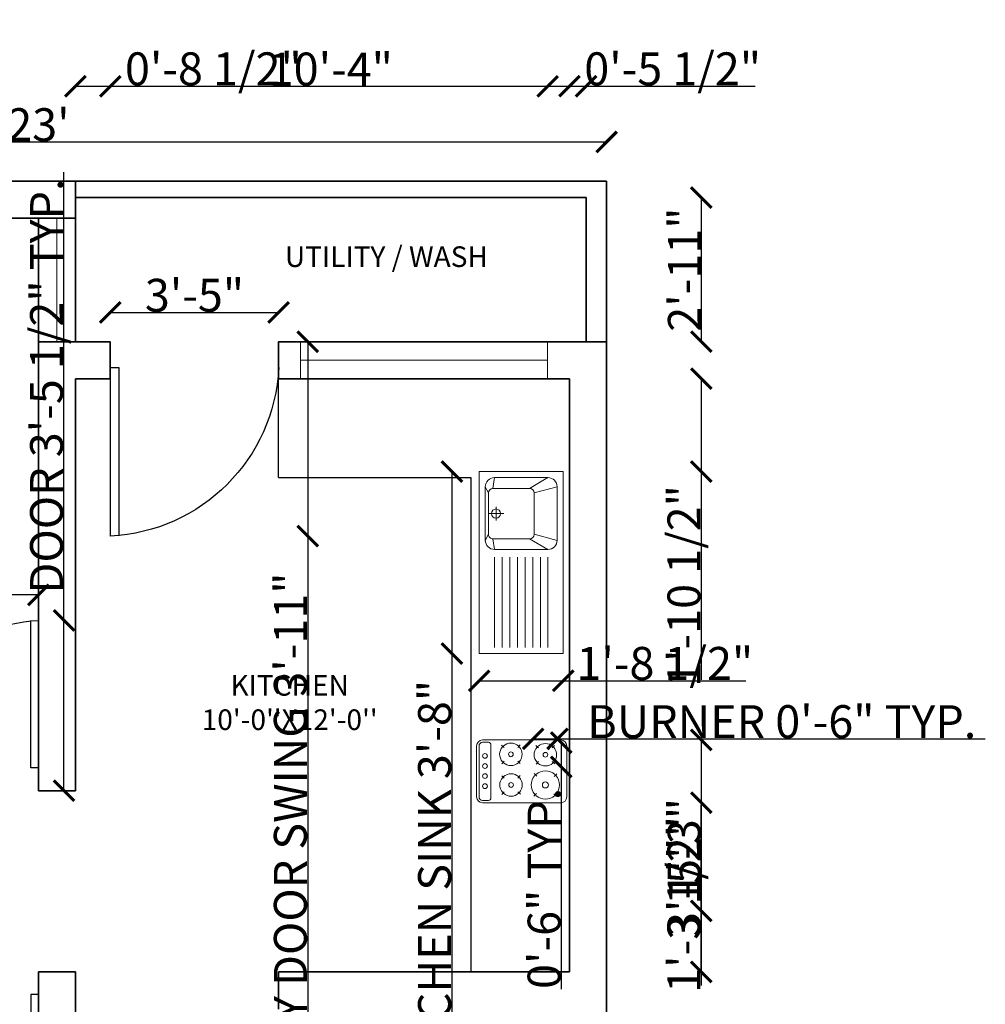
# Model space of a CAD drawing. Units: inches. Extents: x 2435 to 2891, y 1790 to 2334.
# Tile 3 of 3: x 2657 to 2891, y 2052 to 2291. Entities that reach past the tile are written whole.
import ezdxf

# ---------------------------------------------------------------- set-up
doc = ezdxf.new("R2010")
doc.units = ezdxf.units.IN
for name, color, linetype, lineweight in [('A-ANNO-DIMS', 2, 'Continuous', 13), ('A-AREA-IDEN', 7, 'Continuous', 18), ('A-EQPM', 8, 'Continuous', 13), ('A-FLOR-FIXT', 9, 'Continuous', 18), ('DOOR', 30, 'Continuous', 25), ('KITCHEN', 70, 'Continuous', 25), ('WALL', 7, 'Continuous', 35), ('WINDOW', 170, 'Continuous', 18)]:
    doc.layers.add(name, color=color, linetype=linetype, lineweight=lineweight)
doc.styles.get("Standard").update_dxf_attribs({"font": 'arial.ttf'})
doc.dimstyles.get("Standard").update_dxf_attribs({"dimtxt": 8, "dimasz": 5, "dimexe": 0.18, "dimexo": 0.0625, "dimgap": 0.09, "dimtad": 1, "dimdec": 1, "dimzin": 0, "dimdsep": 46, "dimlunit": 4, "dimtxsty": 'Standard', "dimblk": 'ARCHTICK', "dimcen": 0.09, "dimse1": 1, "dimse2": 1, "dimadec": 0, "dimazin": 0, "dimtfac": 1, "dimtdec": 1, "dimtofl": 0, "dimtmove": 0, "dimatfit": 3, "dimfxl": 1, "dimtolj": 1, "dimtzin": 0, "dimarcsym": 0})

# ---------------------------------------------------------------- blocks, each defined once
blk = doc.blocks.new('KK')
for p, q in [((0, 0.55), (0, 0)), ((1.19, 0.55), (0, 0.55)), ((1.19, 0), (1.19, 0.55)), ((0.1, 0.51), (0.14, 0.36)), ((0.45, 0.51), (0.1, 0.51)), ((0.41, 0.36), (0.45, 0.51)), ((0.11, 0.33), (0.04, 0.45)), ((0.04, 0.45), (0.04, 0.1)), ((0.44, 0.33), (0.51, 0.45)), ((0.51, 0.1), (0.51, 0.45)), ((0.56, 0.45), (1.15, 0.45)), ((0.56, 0.4), (1.15, 0.4)), ((0.11, 0.09), (0.11, 0.33)), ((0.14, 0.36), (0.41, 0.36)), ((0.44, 0.33), (0.44, 0.09)), ((0.56, 0.35), (1.15, 0.35)), ((0.56, 0.3), (1.15, 0.3)), ((0.56, 0.25), (1.15, 0.25)), ((0.56, 0.2), (1.15, 0.2)), ((0.275, 0.06), (0.275, 0.16)), ((0.56, 0.15), (1.15, 0.15)), ((0.04, 0.1), (0.11, 0.09)), ((0.23, 0.11), (0.32, 0.11)), ((0.44, 0.09), (0.51, 0.1)), ((0.56, 0.1), (1.15, 0.1)), ((0, 0), (1.19, 0)), ((0.14, 0.06), (0.1, 0.04)), ((0.1, 0.04), (0.45, 0.04)), ((0.41, 0.06), (0.14, 0.06)), ((0.41, 0.06), (0.45, 0.04))]:
    blk.add_line(p, q)
blk.add_circle((0.275, 0.11), 0.03)
for centre, radius, start, end in [((0.1, 0.45), 0.06, 90, 180), ((0.45, 0.45), 0.06, 0, 90), ((0.14, 0.33), 0.03, 90, 180), ((0.41, 0.33), 0.03, 0, 90), ((0.1, 0.1), 0.06, 180, 270), ((0.14, 0.09), 0.03, 180, 270), ((0.41, 0.09), 0.03, 270, 0), ((0.45, 0.1), 0.06, 270, 0)]:
    blk.add_arc(centre, radius, start, end)
blk = doc.blocks.new('AP0B05')
for p, q in [((35, 100), (35, 880)), ((75, 100), (75, 878.9)), ((35, 100), (35, -20)), ((815, 100), (815, -20))]:
    blk.add_line(p, q)
blk.add_lwpolyline([(35, 100), (75, 100)])
blk.add_arc((-2.4, 62.6), 818.3, 2.6212, 87.3788)
blk = doc.blocks.new('_ArchTick')
at = {"color": 0, "linetype": 'ByBlock', "const_width": 0.15}
blk.add_lwpolyline([(-0.5, -0.5), (0.5, 0.5)], dxfattribs=at)
blk = doc.blocks.new('*D10')
at = {"layer": 'A-ANNO-DIMS', "color": 0, "lineweight": -2, "transparency": 16777216}
blk.add_line((2523.44, 2261.69), (2799.44, 2261.69), dxfattribs=at)
at = {"layer": 'Defpoints', "color": 0, "transparency": 16777216}
for p in [(2799.44, 2261.69), (2523.44, 2252.2), (2799.44, 2252.2)]:
    blk.add_point(p, dxfattribs=at)
at = {"layer": 'A-ANNO-DIMS', "color": 0, "lineweight": -2, "transparency": 16777216, "xscale": 5, "yscale": 5, "zscale": 5, "rotation": 180}
blk.add_blockref('_ArchTick', (2523.44, 2261.69), dxfattribs=at)
at = {"layer": 'A-ANNO-DIMS', "color": 0, "lineweight": -2, "transparency": 16777216, "xscale": 5, "yscale": 5, "zscale": 5}
blk.add_blockref('_ArchTick', (2799.44, 2261.69), dxfattribs=at)
at = {"layer": 'A-ANNO-DIMS', "color": 0, "transparency": 16777216, "insert": (2661.44, 2265.87), "char_height": 8, "attachment_point": 5}
blk.add_mtext("\\A1;23'", dxfattribs=at)
blk = doc.blocks.new('WIN-60IN')
blk.add_line((0, 4.5), (60, 4.5))
blk.add_lwpolyline([(0, 9), (60, 9), (60, 0), (0, 0)], close=True)
blk = doc.blocks.new('COOKTOP-BURNER')
for p, q in [((-2.28, 2.23), (-1.67, 1.66)), ((2.23, 2.28), (1.66, 1.67)), ((-2.23, -2.28), (-1.66, -1.67)), ((2.28, -2.23), (1.67, -1.66))]:
    blk.add_line(p, q)
blk.add_circle((0, 0), 0.576)
for start, end in [(48.017, 131.983), (138.017, 221.983), (318.017, 41.983), (228.017, 311.983)]:
    blk.add_arc((0, 0), 2.73, start, end)
blk = doc.blocks.new('*D15')
at = {"layer": 'A-ANNO-DIMS', "color": 0, "lineweight": -2, "transparency": 16777216}
for p, q in [((2667.64, 2145.53), (2667.64, 2254.35)), ((2667.64, 2104.2), (2667.64, 2145.53))]:
    blk.add_line(p, q, dxfattribs=at)
at = {"layer": 'Defpoints', "color": 0, "transparency": 16777216}
for p in [(2661.44, 2145.53), (2667.64, 2145.53), (2661.44, 2104.2)]:
    blk.add_point(p, dxfattribs=at)
at = {"layer": 'A-ANNO-DIMS', "color": 0, "lineweight": -2, "transparency": 16777216, "xscale": 5, "yscale": 5, "zscale": 5}
for p, rotation in [((2667.64, 2145.53), 90), ((2667.64, 2104.2), 270)]:
    blk.add_blockref('_ArchTick', p, dxfattribs=dict(at, rotation=rotation))
at = {"layer": 'A-ANNO-DIMS', "color": 0, "transparency": 16777216, "insert": (2663.41, 2202.44), "char_height": 8, "attachment_point": 5, "rotation": 90}
blk.add_mtext('\\A1;DOOR 3\'-5 1/2" TYP.', dxfattribs=at)
blk = doc.blocks.new('*D16')
at = {"layer": 'A-ANNO-DIMS', "color": 0, "lineweight": -2, "transparency": 16777216}
for p, q in [((2625.63, 2151.73), (2571.69, 2151.73)), ((2661.44, 2151.73), (2625.63, 2151.73))]:
    blk.add_line(p, q, dxfattribs=at)
at = {"layer": 'Defpoints', "color": 0, "transparency": 16777216}
for p in [(2625.63, 2151.73), (2625.63, 2145.53), (2661.44, 2145.53)]:
    blk.add_point(p, dxfattribs=at)
at = {"layer": 'A-ANNO-DIMS', "color": 0, "lineweight": -2, "transparency": 16777216, "xscale": 5, "yscale": 5, "zscale": 5, "rotation": 180}
blk.add_blockref('_ArchTick', (2625.63, 2151.73), dxfattribs=at)
at = {"layer": 'A-ANNO-DIMS', "color": 0, "lineweight": -2, "transparency": 16777216, "xscale": 5, "yscale": 5, "zscale": 5}
blk.add_blockref('_ArchTick', (2661.44, 2151.73), dxfattribs=at)
at = {"layer": 'A-ANNO-DIMS', "color": 0, "transparency": 16777216, "insert": (2596.16, 2155.91), "char_height": 8, "attachment_point": 5}
blk.add_mtext('\\A1;3\'-0" TYP.', dxfattribs=at)
blk = doc.blocks.new('*D17')
at = {"layer": 'A-ANNO-DIMS', "color": 0, "lineweight": -2, "transparency": 16777216}
for p, q in [((2726.86, 2213.2), (2726.86, 2166.02)), ((2726.86, 2166.02), (2726.86, 2011.45))]:
    blk.add_line(p, q, dxfattribs=at)
at = {"layer": 'Defpoints', "color": 0, "transparency": 16777216}
for p in [(2719.78, 2213.2), (2719.78, 2166.02), (2726.86, 2166.02)]:
    blk.add_point(p, dxfattribs=at)
at = {"layer": 'A-ANNO-DIMS', "color": 0, "lineweight": -2, "transparency": 16777216, "xscale": 5, "yscale": 5, "zscale": 5}
for p, rotation in [((2726.86, 2213.2), 90), ((2726.86, 2166.02), 270)]:
    blk.add_blockref('_ArchTick', p, dxfattribs=dict(at, rotation=rotation))
at = {"layer": 'A-ANNO-DIMS', "color": 0, "transparency": 16777216, "insert": (2722.63, 2086.24), "char_height": 8, "attachment_point": 5, "rotation": 90}
blk.add_mtext('\\A1;UTILITY DOOR SWING 3\'-11"', dxfattribs=at)
blk = doc.blocks.new('*D18')
at = {"layer": 'A-ANNO-DIMS', "color": 0, "lineweight": -2, "transparency": 16777216}
blk.add_line((2678.89, 2220.28), (2719.78, 2220.28), dxfattribs=at)
at = {"layer": 'Defpoints', "color": 0, "transparency": 16777216}
for p in [(2719.78, 2220.28), (2678.89, 2213.2), (2719.78, 2213.2)]:
    blk.add_point(p, dxfattribs=at)
at = {"layer": 'A-ANNO-DIMS', "color": 0, "lineweight": -2, "transparency": 16777216, "xscale": 5, "yscale": 5, "zscale": 5, "rotation": 180}
blk.add_blockref('_ArchTick', (2678.89, 2220.28), dxfattribs=at)
at = {"layer": 'A-ANNO-DIMS', "color": 0, "lineweight": -2, "transparency": 16777216, "xscale": 5, "yscale": 5, "zscale": 5}
blk.add_blockref('_ArchTick', (2719.78, 2220.28), dxfattribs=at)
at = {"layer": 'A-ANNO-DIMS', "color": 0, "transparency": 16777216, "insert": (2699.34, 2224.46), "char_height": 8, "attachment_point": 5}
blk.add_mtext('\\A1;3\'-5"', dxfattribs=at)
blk = doc.blocks.new('*D29')
at = {"layer": 'A-ANNO-DIMS', "color": 0, "lineweight": -2, "transparency": 16777216}
for p, q in [((2781.61, 2116.78), (2787.54, 2116.78)), ((2787.54, 2116.78), (2891.43, 2116.78))]:
    blk.add_line(p, q, dxfattribs=at)
at = {"layer": 'Defpoints', "color": 0, "transparency": 16777216}
for p in [(2781.61, 2115.89), (2787.54, 2116.78), (2787.54, 2115.89)]:
    blk.add_point(p, dxfattribs=at)
at = {"layer": 'A-ANNO-DIMS', "color": 0, "lineweight": -2, "transparency": 16777216, "xscale": 5, "yscale": 5, "zscale": 5, "rotation": 180}
blk.add_blockref('_ArchTick', (2781.61, 2116.78), dxfattribs=at)
at = {"layer": 'A-ANNO-DIMS', "color": 0, "lineweight": -2, "transparency": 16777216, "xscale": 5, "yscale": 5, "zscale": 5}
blk.add_blockref('_ArchTick', (2787.54, 2116.78), dxfattribs=at)
at = {"layer": 'A-ANNO-DIMS', "color": 0, "transparency": 16777216, "insert": (2841.99, 2120.96), "char_height": 8, "attachment_point": 5}
blk.add_mtext('\\A1;BURNER 0\'-6" TYP.', dxfattribs=at)
blk = doc.blocks.new('*D30')
at = {"layer": 'A-ANNO-DIMS', "color": 0, "lineweight": -2, "transparency": 16777216}
for p, q in [((2788.43, 2115.89), (2788.43, 2109.96)), ((2788.43, 2109.96), (2788.43, 2056.01))]:
    blk.add_line(p, q, dxfattribs=at)
at = {"layer": 'Defpoints', "color": 0, "transparency": 16777216}
for p in [(2787.54, 2115.89), (2787.54, 2109.96), (2788.43, 2109.96)]:
    blk.add_point(p, dxfattribs=at)
at = {"layer": 'A-ANNO-DIMS', "color": 0, "lineweight": -2, "transparency": 16777216, "xscale": 5, "yscale": 5, "zscale": 5}
for p, rotation in [((2788.43, 2115.89), 90), ((2788.43, 2109.96), 270)]:
    blk.add_blockref('_ArchTick', p, dxfattribs=dict(at, rotation=rotation))
at = {"layer": 'A-ANNO-DIMS', "color": 0, "transparency": 16777216, "insert": (2784.26, 2080.49), "char_height": 8, "attachment_point": 5, "rotation": 90}
blk.add_mtext('\\A1;0\'-6" TYP.', dxfattribs=at)
blk = doc.blocks.new('*D31')
at = {"layer": 'A-ANNO-DIMS', "color": 0, "lineweight": -2, "transparency": 16777216}
for p, q in [((2761.88, 2181.68), (2761.88, 2137.5)), ((2761.88, 2137.5), (2761.88, 2030.06))]:
    blk.add_line(p, q, dxfattribs=at)
at = {"layer": 'Defpoints', "color": 0, "transparency": 16777216}
for p in [(2768.5, 2181.68), (2761.88, 2137.5), (2768.5, 2137.5)]:
    blk.add_point(p, dxfattribs=at)
at = {"layer": 'A-ANNO-DIMS', "color": 0, "lineweight": -2, "transparency": 16777216, "xscale": 5, "yscale": 5, "zscale": 5}
for p, rotation in [((2761.88, 2181.68), 90), ((2761.88, 2137.5), 270)]:
    blk.add_blockref('_ArchTick', p, dxfattribs=dict(at, rotation=rotation))
at = {"layer": 'A-ANNO-DIMS', "color": 0, "transparency": 16777216, "insert": (2757.65, 2081.28), "char_height": 8, "attachment_point": 5, "rotation": 90}
blk.add_mtext('\\A1;KITCHEN SINK 3\'-8"', dxfattribs=at)
blk = doc.blocks.new('*D32')
at = {"layer": 'A-ANNO-DIMS', "color": 0, "lineweight": -2, "transparency": 16777216}
for p, q in [((2768.5, 2130.87), (2788.92, 2130.87)), ((2788.92, 2130.87), (2833.25, 2130.87))]:
    blk.add_line(p, q, dxfattribs=at)
at = {"layer": 'Defpoints', "color": 0, "transparency": 16777216}
for p in [(2768.5, 2137.5), (2788.92, 2137.5), (2788.92, 2130.87)]:
    blk.add_point(p, dxfattribs=at)
at = {"layer": 'A-ANNO-DIMS', "color": 0, "lineweight": -2, "transparency": 16777216, "xscale": 5, "yscale": 5, "zscale": 5, "rotation": 180}
blk.add_blockref('_ArchTick', (2768.5, 2130.87), dxfattribs=at)
at = {"layer": 'A-ANNO-DIMS', "color": 0, "lineweight": -2, "transparency": 16777216, "xscale": 5, "yscale": 5, "zscale": 5}
blk.add_blockref('_ArchTick', (2788.92, 2130.87), dxfattribs=at)
at = {"layer": 'A-ANNO-DIMS', "color": 0, "transparency": 16777216, "insert": (2813.59, 2135.1), "char_height": 8, "attachment_point": 5}
blk.add_mtext('\\A1;1\'-8 1/2"', dxfattribs=at)
blk = doc.blocks.new('*D39')
at = {"layer": 'A-ANNO-DIMS', "color": 0, "lineweight": -2, "transparency": 16777216}
blk.add_line((2670.44, 2275.2), (2794.48, 2275.2), dxfattribs=at)
at = {"layer": 'Defpoints', "color": 0, "transparency": 16777216}
for p in [(2794.48, 2275.2), (2670.44, 2248.2), (2794.48, 2248.2)]:
    blk.add_point(p, dxfattribs=at)
at = {"layer": 'A-ANNO-DIMS', "color": 0, "lineweight": -2, "transparency": 16777216, "xscale": 5, "yscale": 5, "zscale": 5, "rotation": 180}
blk.add_blockref('_ArchTick', (2670.44, 2275.2), dxfattribs=at)
at = {"layer": 'A-ANNO-DIMS', "color": 0, "lineweight": -2, "transparency": 16777216, "xscale": 5, "yscale": 5, "zscale": 5}
blk.add_blockref('_ArchTick', (2794.48, 2275.2), dxfattribs=at)
at = {"layer": 'A-ANNO-DIMS', "color": 0, "transparency": 16777216, "insert": (2732.46, 2279.38), "char_height": 8, "attachment_point": 5}
blk.add_mtext('\\A1;10\'-4"', dxfattribs=at)
blk = doc.blocks.new('*D40')
at = {"layer": 'A-ANNO-DIMS', "color": 0, "lineweight": -2, "transparency": 16777216}
blk.add_line((2822.44, 2248.2), (2822.44, 2213.2), dxfattribs=at)
at = {"layer": 'Defpoints', "color": 0, "transparency": 16777216}
for p in [(2794.48, 2248.2), (2794.48, 2213.2), (2822.44, 2213.2)]:
    blk.add_point(p, dxfattribs=at)
at = {"layer": 'A-ANNO-DIMS', "color": 0, "lineweight": -2, "transparency": 16777216, "xscale": 5, "yscale": 5, "zscale": 5}
for p, rotation in [((2822.44, 2248.2), 90), ((2822.44, 2213.2), 270)]:
    blk.add_blockref('_ArchTick', p, dxfattribs=dict(at, rotation=rotation))
at = {"layer": 'A-ANNO-DIMS', "color": 0, "transparency": 16777216, "insert": (2818.34, 2230.7), "char_height": 8, "attachment_point": 5, "rotation": 90}
blk.add_mtext('\\A1;2\'-11"', dxfattribs=at)
blk = doc.blocks.new('*D46')
at = {"layer": 'A-ANNO-DIMS', "color": 0, "lineweight": -2, "transparency": 16777216}
for p, q in [((2822.44, 2075.04), (2822.44, 2100.73)), ((2822.44, 2060.2), (2822.44, 2075.04))]:
    blk.add_line(p, q, dxfattribs=at)
at = {"layer": 'Defpoints', "color": 0, "transparency": 16777216}
for p in [(2604.44, 2075.04), (2822.44, 2075.04), (2604.44, 2060.2)]:
    blk.add_point(p, dxfattribs=at)
at = {"layer": 'A-ANNO-DIMS', "color": 0, "lineweight": -2, "transparency": 16777216, "xscale": 5, "yscale": 5, "zscale": 5}
for p, rotation in [((2822.44, 2075.04), 90), ((2822.44, 2060.2), 270)]:
    blk.add_blockref('_ArchTick', p, dxfattribs=dict(at, rotation=rotation))
at = {"layer": 'A-ANNO-DIMS', "color": 0, "transparency": 16777216, "insert": (2818.27, 2090.39), "char_height": 8, "attachment_point": 5, "rotation": 90}
blk.add_mtext('\\A1;1\'-3"', dxfattribs=at)
blk = doc.blocks.new('*D47')
at = {"layer": 'A-ANNO-DIMS', "color": 0, "lineweight": -2, "transparency": 16777216}
blk.add_line((2670.44, 1797.2), (2719.78, 1797.2), dxfattribs=at)
at = {"layer": 'Defpoints', "color": 0, "transparency": 16777216}
for p in [(2670.44, 2060.2), (2719.78, 2060.2), (2719.78, 1797.2)]:
    blk.add_point(p, dxfattribs=at)
at = {"layer": 'A-ANNO-DIMS', "color": 0, "lineweight": -2, "transparency": 16777216, "xscale": 5, "yscale": 5, "zscale": 5, "rotation": 180}
blk.add_blockref('_ArchTick', (2670.44, 1797.2), dxfattribs=at)
at = {"layer": 'A-ANNO-DIMS', "color": 0, "lineweight": -2, "transparency": 16777216, "xscale": 5, "yscale": 5, "zscale": 5}
blk.add_blockref('_ArchTick', (2719.78, 1797.2), dxfattribs=at)
at = {"layer": 'A-ANNO-DIMS', "color": 0, "transparency": 16777216, "insert": (2695.11, 1801.43), "char_height": 8, "attachment_point": 5}
blk.add_mtext('\\A1;4\'-1 1/2"', dxfattribs=at)
blk = doc.blocks.new('*D48')
at = {"layer": 'A-ANNO-DIMS', "color": 0, "lineweight": -2, "transparency": 16777216}
blk.add_line((2766.44, 1797.2), (2790.44, 1797.2), dxfattribs=at)
at = {"layer": 'Defpoints', "color": 0, "transparency": 16777216}
for p in [(2766.44, 2060.2), (2790.44, 2060.2), (2790.44, 1797.2)]:
    blk.add_point(p, dxfattribs=at)
at = {"layer": 'A-ANNO-DIMS', "color": 0, "lineweight": -2, "transparency": 16777216, "xscale": 5, "yscale": 5, "zscale": 5, "rotation": 180}
blk.add_blockref('_ArchTick', (2766.44, 1797.2), dxfattribs=at)
at = {"layer": 'A-ANNO-DIMS', "color": 0, "lineweight": -2, "transparency": 16777216, "xscale": 5, "yscale": 5, "zscale": 5}
blk.add_blockref('_ArchTick', (2790.44, 1797.2), dxfattribs=at)
at = {"layer": 'A-ANNO-DIMS', "color": 0, "transparency": 16777216, "insert": (2778.44, 1801.38), "char_height": 8, "attachment_point": 5}
blk.add_mtext('\\A1;2\'-0"', dxfattribs=at)
blk = doc.blocks.new('*D49')
at = {"layer": 'A-ANNO-DIMS', "color": 0, "lineweight": -2, "transparency": 16777216}
for p, q in [((2670.44, 2275.2), (2678.89, 2275.2)), ((2678.89, 2275.2), (2723.98, 2275.2))]:
    blk.add_line(p, q, dxfattribs=at)
at = {"layer": 'Defpoints', "color": 0, "transparency": 16777216}
for p in [(2678.89, 2275.2), (2670.44, 2204.2), (2678.89, 2204.2)]:
    blk.add_point(p, dxfattribs=at)
at = {"layer": 'A-ANNO-DIMS', "color": 0, "lineweight": -2, "transparency": 16777216, "xscale": 5, "yscale": 5, "zscale": 5, "rotation": 180}
blk.add_blockref('_ArchTick', (2670.44, 2275.2), dxfattribs=at)
at = {"layer": 'A-ANNO-DIMS', "color": 0, "lineweight": -2, "transparency": 16777216, "xscale": 5, "yscale": 5, "zscale": 5}
blk.add_blockref('_ArchTick', (2678.89, 2275.2), dxfattribs=at)
at = {"layer": 'A-ANNO-DIMS', "color": 0, "transparency": 16777216, "insert": (2703.93, 2279.43), "char_height": 8, "attachment_point": 5}
blk.add_mtext('\\A1;0\'-8 1/2"', dxfattribs=at)
blk = doc.blocks.new('*D50')
at = {"layer": 'A-ANNO-DIMS', "color": 0, "lineweight": -2, "transparency": 16777216}
for p, q in [((2785.11, 2275.2), (2790.44, 2275.2)), ((2790.44, 2275.2), (2835.53, 2275.2))]:
    blk.add_line(p, q, dxfattribs=at)
at = {"layer": 'Defpoints', "color": 0, "transparency": 16777216}
for p in [(2790.44, 2275.2), (2785.11, 2204.2), (2790.44, 2204.2)]:
    blk.add_point(p, dxfattribs=at)
at = {"layer": 'A-ANNO-DIMS', "color": 0, "lineweight": -2, "transparency": 16777216, "xscale": 5, "yscale": 5, "zscale": 5, "rotation": 180}
blk.add_blockref('_ArchTick', (2785.11, 2275.2), dxfattribs=at)
at = {"layer": 'A-ANNO-DIMS', "color": 0, "lineweight": -2, "transparency": 16777216, "xscale": 5, "yscale": 5, "zscale": 5}
blk.add_blockref('_ArchTick', (2790.44, 2275.2), dxfattribs=at)
at = {"layer": 'A-ANNO-DIMS', "color": 0, "transparency": 16777216, "insert": (2815.49, 2279.43), "char_height": 8, "attachment_point": 5}
blk.add_mtext('\\A1;0\'-5 1/2"', dxfattribs=at)
blk = doc.blocks.new('*D51')
at = {"layer": 'A-ANNO-DIMS', "color": 0, "lineweight": -2, "transparency": 16777216}
for p, q in [((2822.44, 2204.2), (2822.44, 2181.68)), ((2822.44, 2181.68), (2822.44, 2131.13))]:
    blk.add_line(p, q, dxfattribs=at)
at = {"layer": 'Defpoints', "color": 0, "transparency": 16777216}
for p in [(2790.44, 2204.2), (2788.92, 2181.68), (2822.44, 2181.68)]:
    blk.add_point(p, dxfattribs=at)
at = {"layer": 'A-ANNO-DIMS', "color": 0, "lineweight": -2, "transparency": 16777216, "xscale": 5, "yscale": 5, "zscale": 5}
for p, rotation in [((2822.44, 2204.2), 90), ((2822.44, 2181.68), 270)]:
    blk.add_blockref('_ArchTick', p, dxfattribs=dict(at, rotation=rotation))
at = {"layer": 'A-ANNO-DIMS', "color": 0, "transparency": 16777216, "insert": (2818.22, 2153.9), "char_height": 8, "attachment_point": 5, "rotation": 90}
blk.add_mtext('\\A1;1\'-10 1/2"', dxfattribs=at)
blk = doc.blocks.new('*D52')
at = {"layer": 'A-ANNO-DIMS', "color": 0, "lineweight": -2, "transparency": 16777216}
blk.add_line((2822.44, 2101.27), (2822.44, 2060.2), dxfattribs=at)
at = {"layer": 'Defpoints', "color": 0, "transparency": 16777216}
for p in [(2788.32, 2101.27), (2790.44, 2060.2), (2822.44, 2060.2)]:
    blk.add_point(p, dxfattribs=at)
at = {"layer": 'A-ANNO-DIMS', "color": 0, "lineweight": -2, "transparency": 16777216, "xscale": 5, "yscale": 5, "zscale": 5}
for p, rotation in [((2822.44, 2101.27), 90), ((2822.44, 2060.2), 270)]:
    blk.add_blockref('_ArchTick', p, dxfattribs=dict(at, rotation=rotation))
at = {"layer": 'A-ANNO-DIMS', "color": 0, "transparency": 16777216, "insert": (2818.27, 2080.74), "char_height": 8, "attachment_point": 5, "rotation": 90}
blk.add_mtext('\\A1;3\'-5"', dxfattribs=at)
blk = doc.blocks.new('*D53')
at = {"layer": 'A-ANNO-DIMS', "color": 0, "lineweight": -2, "transparency": 16777216}
for p, q in [((2767.88, 1797.2), (2789.76, 1797.2)), ((2789.76, 1797.2), (2821.66, 1797.2))]:
    blk.add_line(p, q, dxfattribs=at)
at = {"layer": 'Defpoints', "color": 0, "transparency": 16777216}
for p in [(2767.88, 2102.71), (2789.76, 2102.71), (2789.76, 1797.2)]:
    blk.add_point(p, dxfattribs=at)
at = {"layer": 'A-ANNO-DIMS', "color": 0, "lineweight": -2, "transparency": 16777216, "xscale": 5, "yscale": 5, "zscale": 5, "rotation": 180}
blk.add_blockref('_ArchTick', (2767.88, 1797.2), dxfattribs=at)
at = {"layer": 'A-ANNO-DIMS', "color": 0, "lineweight": -2, "transparency": 16777216, "xscale": 5, "yscale": 5, "zscale": 5}
blk.add_blockref('_ArchTick', (2789.76, 1797.2), dxfattribs=at)
at = {"layer": 'A-ANNO-DIMS', "color": 0, "transparency": 16777216, "insert": (2808.21, 1801.38), "char_height": 8, "attachment_point": 5}
blk.add_mtext('\\A1;1\'-10"', dxfattribs=at)
blk = doc.blocks.new('*D54')
at = {"layer": 'A-ANNO-DIMS', "color": 0, "lineweight": -2, "transparency": 16777216}
for p, q in [((2822.44, 2116.52), (2822.44, 2101.27)), ((2822.44, 2101.27), (2822.44, 2056.94))]:
    blk.add_line(p, q, dxfattribs=at)
at = {"layer": 'Defpoints', "color": 0, "transparency": 16777216}
for p in [(2788.32, 2116.52), (2788.32, 2101.27), (2822.44, 2101.27)]:
    blk.add_point(p, dxfattribs=at)
at = {"layer": 'A-ANNO-DIMS', "color": 0, "lineweight": -2, "transparency": 16777216, "xscale": 5, "yscale": 5, "zscale": 5}
for p, rotation in [((2822.44, 2116.52), 90), ((2822.44, 2101.27), 270)]:
    blk.add_blockref('_ArchTick', p, dxfattribs=dict(at, rotation=rotation))
at = {"layer": 'A-ANNO-DIMS', "color": 0, "transparency": 16777216, "insert": (2818.22, 2076.6), "char_height": 8, "attachment_point": 5, "rotation": 90}
blk.add_mtext('\\A1;1\'-3 1/2"', dxfattribs=at)

msp = doc.modelspace()

# ---------------------------------------------------------------- linework, layer by layer
at = {"layer": 'A-EQPM'}
for p, q in [((2788.32, 2116.52), (2769.32, 2116.52)), ((2770.76, 2115.95), (2769.32, 2115.95)), ((2771.34, 2102.42), (2771.34, 2115.37)), ((2767.88, 2115.08), (2767.88, 2102.71)), ((2768.46, 2115.08), (2768.46, 2102.71)), ((2789.76, 2102.71), (2789.76, 2115.08)), ((2781.87, 2108.39), (2782.51, 2107.71)), ((2787.38, 2108.29), (2786.7, 2107.65)), ((2773.96, 2107.83), (2774.56, 2107.23)), ((2778.48, 2107.86), (2777.87, 2107.25)), ((2773.98, 2103.31), (2774.58, 2103.92)), ((2778.5, 2103.34), (2777.89, 2103.94)), ((2781.77, 2102.89), (2782.45, 2103.52)), ((2787.28, 2102.78), (2786.64, 2103.46)), ((2769.32, 2101.85), (2770.76, 2101.85)), ((2769.32, 2101.27), (2788.32, 2101.27))]:
    msp.add_line(p, q, dxfattribs=at)
for centre, radius in [((2769.9, 2112.64), 0.576), ((2769.9, 2110.19), 0.576), ((2769.9, 2107.75), 0.576), ((2769.9, 2105.3), 0.576), ((2776.23, 2105.59), 0.576), ((2784.57, 2105.59), 0.722)]:
    msp.add_circle(centre, radius, dxfattribs=at)
for centre, radius, start, end in [((2769.32, 2115.08), 1.44, 90, 180), ((2769.32, 2115.08), 0.863, 90, 180), ((2770.76, 2115.37), 0.576, 0, 90), ((2788.32, 2115.08), 1.44, 0, 90), ((2776.23, 2105.59), 2.73, 48.017, 131.983), ((2784.57, 2105.59), 3.43, 48.017, 131.983), ((2776.23, 2105.59), 2.73, 138.017, 221.983), ((2776.23, 2105.59), 2.73, 318.017, 41.983), ((2784.57, 2105.59), 3.43, 138.017, 221.983), ((2784.57, 2105.59), 3.43, 318.017, 41.983), ((2776.23, 2105.59), 2.73, 228.017, 311.983), ((2769.32, 2102.71), 1.44, 180, 270), ((2769.32, 2102.71), 0.863, 180, 270), ((2770.76, 2102.42), 0.576, 270, 0), ((2784.57, 2105.59), 3.43, 228.017, 311.983), ((2788.32, 2102.71), 1.44, 270, 0)]:
    msp.add_arc(centre, radius, start, end, dxfattribs=at)
at = {"layer": 'KITCHEN'}
for p, q in [((2719.78, 2180.2), (2719.78, 2204.2)), ((2719.78, 2180.2), (2766.44, 2180.2)), ((2766.44, 2180.2), (2766.44, 2060.2))]:
    msp.add_line(p, q, dxfattribs=at)
at = {"layer": 'WALL'}
for p, q in [((2523.44, 2252.2), (2799.44, 2252.2)), ((2670.44, 2252.2), (2670.44, 2213.2)), ((2799.44, 2252.2), (2799.44, 1820.2)), ((2670.44, 2248.2), (2794.48, 2248.2)), ((2794.48, 2248.2), (2794.48, 2213.2)), ((2532.44, 2243.2), (2670.44, 2243.2)), ((2661.44, 2243.2), (2661.44, 2104.2)), ((2661.44, 2213.2), (2678.89, 2213.2)), ((2678.89, 2213.2), (2678.89, 2204.2)), ((2719.78, 2213.2), (2719.78, 2204.2)), ((2719.78, 2213.2), (2799.44, 2213.2)), ((2670.44, 2204.2), (2670.44, 2104.2)), ((2670.44, 2204.2), (2678.89, 2204.2)), ((2719.78, 2204.2), (2790.44, 2204.2)), ((2790.44, 2204.2), (2790.44, 2060.2)), ((2661.44, 2104.2), (2670.44, 2104.2)), ((2661.44, 2060.2), (2661.44, 1901.2)), ((2661.44, 2060.2), (2670.44, 2060.2)), ((2670.44, 2060.2), (2670.44, 1901.2)), ((2719.78, 2060.2), (2719.78, 2051.2)), ((2719.78, 2060.2), (2790.44, 2060.2))]:
    msp.add_line(p, q, dxfattribs=at)
at = {"layer": 'WINDOW'}
msp.add_line((2665.94, 2213.2), (2665.94, 2243.2), dxfattribs=at)
msp.add_lwpolyline([(2661.44, 2213.2), (2661.44, 2243.2), (2670.44, 2243.2), (2670.44, 2213.2)], close=True, dxfattribs=at)

# ---------------------------------------------------------------- block references
at = {"layer": 'A-EQPM'}
msp.add_blockref('COOKTOP-BURNER', (2776.19, 2113.03), dxfattribs=at)
at = {"layer": 'A-EQPM', "rotation": 270.0000000002154}
msp.add_blockref('COOKTOP-BURNER', (2784.57, 2112.93), dxfattribs=at)
at = {"layer": 'A-FLOR-FIXT', "xscale": 37.12264446484568, "yscale": 37.12264446484568, "zscale": 37.12264446484568, "rotation": 270}
msp.add_blockref('KK', (2768.5, 2181.68), dxfattribs=at)
at = {"layer": 'DOOR', "rotation": 180}
for p, xscale, yscale, zscale in [((2677.06, 2212.16), -0.05242749672078, 0.05242749672078, 0.05242749672078), ((2663.05, 2059.29), 0.0459165349072538, 0.0459165349072538, 0.0459165349072538)]:
    msp.add_blockref('AP0B05', p, dxfattribs=dict(at, xscale=xscale, yscale=yscale, zscale=zscale))
at = {"layer": 'DOOR', "xscale": -0.0459165349072543, "yscale": 0.0459165349072543, "zscale": 0.0459165349072543}
msp.add_blockref('AP0B05', (2663.05, 2105.12), dxfattribs=at)
at = {"layer": 'WINDOW'}
msp.add_blockref('WIN-60IN', (2725.11, 2204.2), dxfattribs=at)

# ---------------------------------------------------------------- texts
at = {"layer": 'A-AREA-IDEN', "char_height": 5, "attachment_point": 1}
for s, width, insert in [('\\pxqc;UTILITY / WASH', 56.0393, (2717.93, 2236.33)), ("\\pxqc;KITCHEN\\P10'-0''X12'-0''", 37.2819, (2703.82, 2132.27))]:
    msp.add_mtext_dynamic_manual_height_columns(s, width=width, gutter_width=12.5, heights=[0], dxfattribs=dict(at, insert=insert))

# ---------------------------------------------------------------- dimensions: what is measured, and where the dimension line sits
at = {"layer": 'A-ANNO-DIMS'}
for base, p1, p2, override, picture, middle in [((2678.8908, 2275.2042), (2670.4449, 2204.2042), (2678.8908, 2204.2042), {"dimdec": 1, "dimlfac": 1, "dimrnd": 0, "dimzin": 1, "dimdsep": 46, "dimlunit": 4, "dimfrac": 2}, '*D49', (2703.9344, 2279.4306)), ((2790.44, 2275.2), (2785.11, 2204.2), (2790.44, 2204.2), {"dimdec": 1, "dimlfac": 1, "dimrnd": 0, "dimzin": 1, "dimdsep": 46, "dimlunit": 4, "dimfrac": 2}, '*D50', (2815.49, 2279.43)), ((2794.48, 2275.2), (2670.44, 2248.2), (2794.48, 2248.2), {"dimdec": 1, "dimlfac": 1, "dimrnd": 0, "dimzin": 1, "dimdsep": 46, "dimlunit": 4, "dimfrac": 2}, '*D39', (2732.46, 2279.38)), ((2799.44, 2261.69), (2523.44, 2252.2), (2799.44, 2252.2), {"dimclrd": 0, "dimclre": 0, "dimclrt": 0}, '*D10', (2661.44, 2265.87)), ((2719.78, 2220.28), (2678.89, 2213.2), (2719.78, 2213.2), {"dimdec": 1, "dimlfac": 1, "dimrnd": 0, "dimzin": 1, "dimdsep": 46, "dimlunit": 4, "dimfrac": 2}, '*D18', (2699.34, 2224.46)), ((2788.92, 2130.87), (2768.5, 2137.5), (2788.92, 2137.5), {"dimdec": 1, "dimlfac": 1, "dimrnd": 0, "dimzin": 1, "dimdsep": 46, "dimlunit": 4, "dimfrac": 2}, '*D32', (2813.59, 2135.1)), ((2789.76, 1797.2), (2767.88, 2102.71), (2789.76, 2102.71), {"dimdec": 1, "dimlfac": 1, "dimrnd": 0, "dimzin": 1, "dimdsep": 46, "dimlunit": 4, "dimfrac": 2}, '*D53', (2808.21, 1801.38)), ((2719.78, 1797.2), (2670.44, 2060.2), (2719.78, 2060.2), {"dimdec": 1, "dimlfac": 1, "dimrnd": 0, "dimzin": 1, "dimdsep": 46, "dimlunit": 4, "dimfrac": 2}, '*D47', (2695.11, 1801.43)), ((2790.44, 1797.2), (2766.44, 2060.2), (2790.44, 2060.2), {"dimdec": 1, "dimlfac": 1, "dimrnd": 0, "dimzin": 1, "dimdsep": 46, "dimlunit": 4, "dimfrac": 2}, '*D48', (2778.44, 1801.38))]:
    dim = msp.add_linear_dim(base=base, p1=p1, p2=p2, dimstyle='Standard', override=override, dxfattribs=at)
    dim.commit()
    dim.dimension.update_dxf_attribs({"geometry": picture, "text_midpoint": middle})
for base, p1, p2, angle, text, picture, middle in [((2667.64, 2145.53), (2661.44, 2104.2), (2661.44, 2145.53), 90, 'DOOR <> TYP.', '*D15', (2663.41, 2202.44)), ((2726.86, 2166.02), (2719.78, 2213.2), (2719.78, 2166.02), 270, 'UTILITY DOOR SWING <>', '*D17', (2722.63, 2086.24)), ((2761.88, 2137.5), (2768.5, 2181.68), (2768.5, 2137.5), 270, 'KITCHEN SINK <>', '*D31', (2757.65, 2081.28)), ((2625.63, 2151.73), (2661.44, 2145.53), (2625.63, 2145.53), 180, '<> TYP.', '*D16', (2596.16, 2155.91)), ((2787.54, 2116.78), (2781.61, 2115.89), (2787.54, 2115.89), 0, 'BURNER <> TYP.', '*D29', (2841.99, 2120.96)), ((2788.43, 2109.96), (2787.54, 2115.89), (2787.54, 2109.96), 270, '<> TYP.', '*D30', (2784.26, 2080.49))]:
    dim = msp.add_linear_dim(base=base, p1=p1, p2=p2, angle=angle, text=text, dimstyle='Standard', override={"dimdec": 1, "dimlfac": 1, "dimrnd": 0, "dimzin": 1, "dimdsep": 46, "dimlunit": 4, "dimfrac": 2}, dxfattribs=at)
    dim.commit()
    dim.dimension.update_dxf_attribs({"geometry": picture, "text_midpoint": middle})
for base, p1, p2, picture, middle in [((2822.44, 2213.2), (2794.48, 2248.2), (2794.48, 2213.2), '*D40', (2818.34, 2230.7)), ((2822.44, 2181.68), (2790.44, 2204.2), (2788.92, 2181.68), '*D51', (2818.22, 2153.9)), ((2822.4449, 2101.2704), (2788.3163, 2116.5237), (2788.3163, 2101.2704), '*D54', (2818.2158, 2076.6034)), ((2822.44, 2060.2), (2788.32, 2101.27), (2790.44, 2060.2), '*D52', (2818.27, 2080.74)), ((2822.44, 2075.04), (2604.44, 2060.2), (2604.44, 2075.04), '*D46', (2818.27, 2090.39))]:
    dim = msp.add_linear_dim(base=base, p1=p1, p2=p2, angle=90, dimstyle='Standard', override={"dimdec": 1, "dimlfac": 1, "dimrnd": 0, "dimzin": 1, "dimdsep": 46, "dimlunit": 4, "dimfrac": 2}, dxfattribs=at)
    dim.commit()
    dim.dimension.update_dxf_attribs({"geometry": picture, "text_midpoint": middle})

doc.saveas('drawing.dxf')
